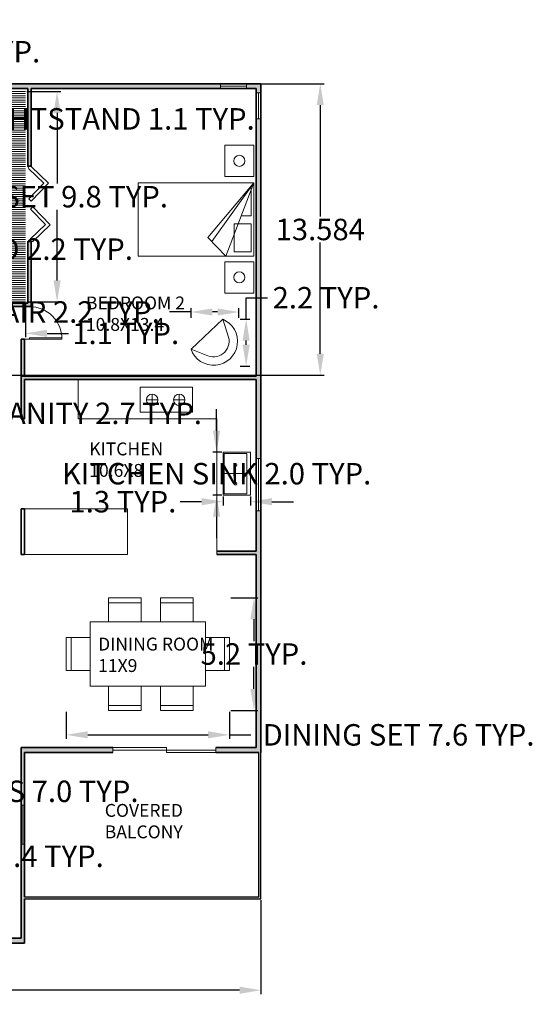
# Model space of a CAD drawing. Units: metres. Extents: x 25.1 to 96.1, y 24.3 to 71.3.
# Tile 5 of 5: x 72.2 to 96.1, y 24.9 to 70.8. Entities that reach past the tile are written whole.
import ezdxf

# ---------------------------------------------------------------- set-up
doc = ezdxf.new("R2010")
doc.units = ezdxf.units.M
doc.header["$MEASUREMENT"] = 0
for name, color, linetype, lineweight in [('A-AREA-IDEN', 1, 'Continuous', 18), ('A-EQPM', 163, 'Continuous', 18), ('A-FLOR-CASE', 8, 'Continuous', 18), ('A-FLOR-FIXT', 163, 'Continuous', 18), ('A-FLOR-RAIL', 7, 'Continuous', 25), ('A-GLAZ', 4, 'Continuous', 18), ('A-WALL', 7, 'Continuous', 35), ('A-WALL-PATT', 252, 'Continuous', 13), ('dimension', 80, 'Continuous', 18), ('door', 17, 'Continuous', 18), ('furniture', 163, 'Continuous', 18)]:
    doc.layers.add(name, color=color, linetype=linetype, lineweight=lineweight)
doc.styles.get("Standard").update_dxf_attribs({"font": 'arial.ttf'})
doc.dimstyles.get("Standard").update_dxf_attribs({"dimtxt": 1, "dimasz": 1, "dimexe": 0.18, "dimexo": 0.0625, "dimgap": 0.09, "dimtad": 0, "dimtih": 1, "dimtoh": 1, "dimdec": 1, "dimzin": 0, "dimdsep": 46, "dimtxsty": 'Standard', "dimcen": 0.09, "dimadec": 0, "dimazin": 0, "dimtfac": 1, "dimtdec": 1, "dimtofl": 0, "dimtmove": 0, "dimatfit": 3, "dimfxl": 1, "dimtolj": 1, "dimtzin": 0, "dimarcsym": 0})

# ---------------------------------------------------------------- blocks, each defined once
blk = doc.blocks.new('sink')
for points in [[(16.263, 3.026), (17.543, 3.026), (17.543, 1.019), (16.263, 1.019)], [(17.495, 2.968), (16.431, 2.968), (16.431, 2.028), (17.495, 2.028)], [(17.495, 2.028), (16.431, 2.028), (16.431, 1.081), (17.495, 1.081)]]:
    blk.add_lwpolyline(points, close=True)
for centre in [(16.963, 2.431), (16.961, 1.556)]:
    blk.add_circle(centre, 0.0675)
blk = doc.blocks.new('gas')
for p, q in [((20.28, 5.991), (20.28, 5.463)), ((21.546, 5.991), (21.546, 5.463)), ((20.016, 5.727), (20.544, 5.727)), ((21.282, 5.727), (21.81, 5.727))]:
    blk.add_line(p, q)
blk.add_lwpolyline([(19.729, 6.31), (22.157, 6.31), (22.157, 5.155), (19.729, 5.155)], close=True)
for centre in [(20.28, 5.727), (21.546, 5.727)]:
    blk.add_circle(centre, 0.264)
blk = doc.blocks.new('b')
for p, q in [((16.374, 15.368), (18.513, 12.83)), ((17.666, 11.96), (16.374, 15.368)), ((16.374, 15.368), (18.324, 12.637)), ((18.513, 12.83), (17.666, 11.96))]:
    blk.add_line(p, q)
for points in [[(16.362, 17.126), (17.718, 17.126), (17.718, 15.669), (16.362, 15.669)], [(16.374, 15.368), (21.762, 15.368), (21.762, 11.96), (16.374, 11.96)], [(16.486, 12.161), (17.289, 12.161), (17.289, 13.464), (16.486, 13.464)], [(16.362, 11.698), (17.718, 11.698), (17.718, 10.242), (16.362, 10.242)]]:
    blk.add_lwpolyline(points, close=True)
blk.add_lwpolyline([(16.564, 15.144), (16.486, 15.144), (16.486, 13.84), (16.953, 13.84)])
for centre in [(17.04, 16.398), (17.04, 10.97)]:
    blk.add_circle(centre, 0.259)
blk = doc.blocks.new('cc')
for p, q in [((17.83, 9.22), (17.545, 8.337)), ((17.83, 9.22), (19.307, 7.829)), ((19.307, 7.829), (18.516, 7.517))]:
    blk.add_line(p, q)
for radius, start, end in [(1.115, 112.1788, 341.2424), (0.721, 156.2062, 291.5475)]:
    blk.add_arc((18.251, 8.188), radius, start, end)
blk = doc.blocks.new('d')
for p, q in [((25.537, 16.335), (24.732, 15.559)), ((25.644, 16.224), (24.951, 15.555)), ((25.537, 16.335), (25.687, 16.335)), ((25.644, 16.224), (25.687, 16.335)), ((24.732, 15.559), (25.537, 14.725)), ((24.951, 15.555), (25.648, 14.833)), ((25.648, 14.833), (25.537, 14.725))]:
    blk.add_line(p, q)
blk = doc.blocks.new('f')
at = {"layer": 'furniture'}
for p, q in [((25.769, 19.917), (26.843, 19.917)), ((25.769, 19.817), (26.843, 19.817)), ((25.769, 19.717), (26.843, 19.717)), ((25.769, 19.617), (26.843, 19.617)), ((25.769, 19.517), (26.843, 19.517)), ((25.769, 19.417), (26.843, 19.417)), ((25.769, 19.317), (26.843, 19.317)), ((25.769, 19.217), (26.843, 19.217)), ((25.769, 19.117), (26.843, 19.117)), ((25.769, 19.017), (26.843, 19.017)), ((25.769, 18.917), (26.843, 18.917)), ((25.769, 18.817), (26.843, 18.817)), ((25.769, 18.717), (26.843, 18.717)), ((25.769, 18.617), (26.843, 18.617)), ((25.769, 18.517), (26.843, 18.517)), ((25.769, 18.417), (26.843, 18.417)), ((25.769, 18.317), (26.843, 18.317)), ((25.769, 18.217), (26.843, 18.217)), ((25.769, 18.117), (26.843, 18.117)), ((25.769, 18.017), (26.843, 18.017)), ((25.769, 17.917), (26.843, 17.917)), ((25.769, 17.817), (26.843, 17.817)), ((25.769, 17.717), (26.843, 17.717)), ((25.769, 17.617), (26.843, 17.617)), ((25.769, 17.517), (26.843, 17.517)), ((25.769, 17.417), (26.843, 17.417)), ((25.769, 17.317), (26.843, 17.317)), ((25.769, 17.217), (26.843, 17.217)), ((25.769, 17.117), (26.843, 17.117)), ((25.769, 17.017), (26.843, 17.017)), ((25.769, 16.917), (26.843, 16.917)), ((25.769, 16.817), (26.843, 16.817)), ((25.769, 16.717), (26.843, 16.717)), ((25.769, 16.617), (26.843, 16.617)), ((25.769, 16.517), (26.843, 16.517)), ((25.769, 16.417), (26.843, 16.417)), ((25.769, 16.317), (26.843, 16.317)), ((25.769, 16.217), (26.843, 16.217)), ((25.769, 16.117), (26.843, 16.117)), ((25.769, 16.017), (26.843, 16.017)), ((25.769, 15.917), (26.843, 15.917)), ((25.769, 15.817), (26.843, 15.817)), ((25.769, 15.717), (26.843, 15.717)), ((25.769, 15.617), (26.843, 15.617)), ((25.769, 15.517), (26.843, 15.517)), ((25.769, 15.417), (26.843, 15.417)), ((25.769, 15.317), (26.843, 15.317)), ((25.769, 15.217), (26.843, 15.217)), ((25.769, 15.117), (26.843, 15.117)), ((25.769, 15.017), (26.843, 15.017)), ((25.769, 14.917), (26.843, 14.917)), ((25.769, 14.817), (26.843, 14.817)), ((25.769, 14.717), (26.843, 14.717)), ((25.769, 14.617), (26.843, 14.617)), ((25.769, 14.517), (26.843, 14.517)), ((25.769, 14.417), (26.843, 14.417)), ((25.769, 14.317), (26.843, 14.317)), ((25.769, 14.217), (26.843, 14.217)), ((25.769, 14.117), (26.843, 14.117)), ((25.769, 14.017), (26.843, 14.017)), ((25.769, 13.917), (26.843, 13.917)), ((25.769, 13.817), (26.843, 13.817)), ((25.769, 13.717), (26.843, 13.717)), ((25.769, 13.617), (26.843, 13.617)), ((25.769, 13.517), (26.843, 13.517)), ((25.769, 13.417), (26.843, 13.417)), ((25.769, 13.317), (26.843, 13.317)), ((25.769, 13.217), (26.843, 13.217)), ((25.769, 13.117), (26.843, 13.117)), ((25.769, 13.017), (26.843, 13.017)), ((25.769, 12.917), (26.843, 12.917)), ((25.769, 12.817), (26.843, 12.817)), ((25.769, 12.717), (26.843, 12.717)), ((25.769, 12.617), (26.843, 12.617)), ((25.769, 12.517), (26.843, 12.517)), ((25.769, 12.417), (26.843, 12.417)), ((25.769, 12.317), (26.843, 12.317)), ((25.769, 12.217), (26.843, 12.217)), ((25.769, 12.117), (26.843, 12.117)), ((25.769, 12.017), (26.843, 12.017)), ((25.769, 11.917), (26.843, 11.917)), ((25.769, 11.817), (26.843, 11.817)), ((25.769, 11.717), (26.843, 11.717)), ((25.769, 11.617), (26.843, 11.617)), ((25.769, 11.517), (26.843, 11.517)), ((25.769, 11.417), (26.843, 11.417)), ((25.769, 11.317), (26.843, 11.317)), ((25.769, 11.217), (26.843, 11.217)), ((25.769, 11.117), (26.843, 11.117)), ((25.769, 11.017), (26.843, 11.017)), ((25.769, 10.917), (26.843, 10.917)), ((25.769, 10.817), (26.843, 10.817)), ((25.769, 10.717), (26.843, 10.717)), ((25.769, 10.617), (26.843, 10.617)), ((25.769, 10.517), (26.843, 10.517)), ((25.769, 10.417), (26.843, 10.417)), ((25.769, 10.317), (26.843, 10.317)), ((25.769, 10.217), (26.843, 10.217)), ((25.769, 10.117), (26.843, 10.117))]:
    blk.add_line(p, q, dxfattribs=at)
blk = doc.blocks.new('*U22')
for p, q in [((0, 0), (0, -6)), ((40, 0), (40, -6))]:
    blk.add_line(p, q)
blk.add_lwpolyline([(0, 0), (0, 40), (1.75, 40), (1.75, 0)], close=True)
blk.add_arc((0, 0), 40, 0, 90)
blk = doc.blocks.new('tttt')
for points in [[(21.475, -3.758), (19.715, -3.758), (19.715, -3.49), (21.475, -3.49)], [(24.267, -3.758), (22.507, -3.758), (22.507, -3.49), (24.267, -3.49)], [(19.715, -4.78), (21.475, -4.78), (21.475, -3.758), (19.715, -3.758)], [(22.507, -4.78), (24.267, -4.78), (24.267, -3.758), (22.507, -3.758)], [(18.746, -4.78), (24.929, -4.78), (24.929, -8.239), (18.746, -8.239)], [(17.724, -5.63), (17.724, -7.389), (17.456, -7.389), (17.456, -5.63)], [(18.746, -7.389), (18.746, -5.63), (17.724, -5.63), (17.724, -7.389)], [(24.929, -7.389), (24.929, -5.63), (25.951, -5.63), (25.951, -7.389)], [(25.951, -5.63), (25.951, -7.389), (26.219, -7.389), (26.219, -5.63)], [(19.715, -8.239), (21.475, -8.239), (21.475, -9.262), (19.715, -9.262)], [(22.507, -8.239), (24.267, -8.239), (24.267, -9.262), (22.507, -9.262)], [(21.475, -9.262), (19.715, -9.262), (19.715, -9.529), (21.475, -9.529)], [(24.267, -9.262), (22.507, -9.262), (22.507, -9.529), (24.267, -9.529)]]:
    blk.add_lwpolyline(points, close=True)
blk = doc.blocks.new('*D24')
at = {"layer": 'Defpoints', "color": 0, "transparency": 16777216}
for p in [(31.99, 29.798), (83.411, 29.798), (83.411, 25.547)]:
    blk.add_point(p, dxfattribs=at)
at = {"layer": 'dimension', "color": 0, "lineweight": -2, "transparency": 16777216}
for p, q in [((31.99, 29.735), (31.99, 25.367)), ((83.411, 29.735), (83.411, 25.367)), ((32.99, 25.547), (56.314, 25.547)), ((82.411, 25.547), (59.087, 25.547))]:
    blk.add_line(p, q, dxfattribs=at)
at = {"layer": 'dimension', "color": 0, "transparency": 16777216}
for points in [[(32.99, 25.713), (32.99, 25.38), (31.99, 25.547)], [(82.411, 25.713), (82.411, 25.38), (83.411, 25.547)]]:
    blk.add_solid(points, dxfattribs=at)
at = {"layer": 'dimension', "color": 0, "transparency": 16777216, "insert": (57.7, 25.547), "char_height": 1, "attachment_point": 5}
blk.add_mtext('\\A1;51.4', dxfattribs=at)
blk = doc.blocks.new('DOOR-BALCONY-SLIDING')
for p, q in [((0, 0.23), (2.501, 0.23)), ((2.501, 0.23), (2.501, 0)), ((2.501, 0), (4.797, 0))]:
    blk.add_line(p, q)
blk.add_lwpolyline([(4.797, 0.115), (4.797, 0.115), (0, 0.115), (0, 0.115)])
blk = doc.blocks.new('*D36')
at = {"layer": 'Defpoints', "color": 0, "transparency": 16777216}
for p in [(72.431, 67.419), (73.901, 67.419), (72.431, 57.619)]:
    blk.add_point(p, dxfattribs=at)
at = {"layer": 'dimension', "color": 0, "lineweight": -2, "transparency": 16777216}
for p, q in [((72.494, 67.419), (74.081, 67.419)), ((73.901, 66.419), (73.901, 63.126)), ((73.901, 58.619), (73.901, 61.912)), ((72.494, 57.619), (74.081, 57.619))]:
    blk.add_line(p, q, dxfattribs=at)
at = {"layer": 'dimension', "color": 0, "transparency": 16777216}
for points in [[(73.735, 66.419), (74.068, 66.419), (73.901, 67.419)], [(73.735, 58.619), (74.068, 58.619), (73.901, 57.619)]]:
    blk.add_solid(points, dxfattribs=at)
at = {"layer": 'dimension', "color": 0, "transparency": 16777216, "insert": (73.901, 62.519), "char_height": 1, "attachment_point": 5}
blk.add_mtext('\\A1;CLOSET 9.8 TYP.', dxfattribs=at)
blk = doc.blocks.new('*D37')
at = {"layer": 'Defpoints', "color": 0, "transparency": 16777216}
for p in [(71.357, 57.619), (72.431, 57.619), (72.431, 56.149)]:
    blk.add_point(p, dxfattribs=at)
at = {"layer": 'dimension', "color": 0, "lineweight": -2, "transparency": 16777216}
for p, q in [((71.357, 57.557), (71.357, 55.969)), ((72.431, 57.557), (72.431, 55.969)), ((70.357, 56.149), (69.357, 56.149)), ((73.431, 56.149), (74.431, 56.149))]:
    blk.add_line(p, q, dxfattribs=at)
at = {"layer": 'dimension', "color": 0, "transparency": 16777216}
for points in [[(70.357, 56.316), (70.357, 55.982), (71.357, 56.149)], [(73.431, 56.316), (73.431, 55.982), (72.431, 56.149)]]:
    blk.add_solid(points, dxfattribs=at)
at = {"layer": 'dimension', "color": 0, "transparency": 16777216, "insert": (77.102, 56.149), "char_height": 1, "attachment_point": 5}
blk.add_mtext('\\A1;1.1 TYP.', dxfattribs=at)
blk = doc.blocks.new('*D39')
at = {"layer": 'Defpoints', "color": 0, "transparency": 16777216}
for p in [(69.103, 30.788), (69.861, 30.788), (69.103, 28.392)]:
    blk.add_point(p, dxfattribs=at)
at = {"layer": 'dimension', "color": 0, "lineweight": -2, "transparency": 16777216}
for p, q in [((69.861, 30.788), (69.861, 31.788)), ((69.861, 31.788), (70.861, 31.788)), ((69.166, 30.788), (70.041, 30.788)), ((69.861, 29.392), (69.861, 29.788)), ((69.166, 28.392), (70.041, 28.392))]:
    blk.add_line(p, q, dxfattribs=at)
at = {"layer": 'dimension', "color": 0, "transparency": 16777216}
for points in [[(69.694, 29.788), (70.027, 29.788), (69.861, 30.788)], [(69.694, 29.392), (70.027, 29.392), (69.861, 28.392)]]:
    blk.add_solid(points, dxfattribs=at)
at = {"layer": 'dimension', "color": 0, "transparency": 16777216, "insert": (73.587, 31.788), "char_height": 1, "attachment_point": 5}
blk.add_mtext('\\A1;2.4 TYP.', dxfattribs=at)
blk = doc.blocks.new('*D42')
at = {"layer": 'Defpoints', "color": 0, "transparency": 16777216}
for p in [(81.341, 50.616), (81.642, 50.616), (81.642, 48.609)]:
    blk.add_point(p, dxfattribs=at)
at = {"layer": 'dimension', "color": 0, "lineweight": -2, "transparency": 16777216}
for p, q in [((81.341, 51.616), (81.341, 52.616)), ((81.579, 50.616), (81.161, 50.616)), ((81.579, 48.609), (81.161, 48.609)), ((81.341, 47.609), (81.341, 46.609))]:
    blk.add_line(p, q, dxfattribs=at)
at = {"layer": 'dimension', "color": 0, "transparency": 16777216}
for points in [[(81.174, 51.616), (81.507, 51.616), (81.341, 50.616)], [(81.174, 47.609), (81.507, 47.609), (81.341, 48.609)]]:
    blk.add_solid(points, dxfattribs=at)
at = {"layer": 'dimension', "color": 0, "transparency": 16777216, "insert": (81.341, 49.612), "char_height": 1, "attachment_point": 5}
blk.add_mtext('\\A1;KITCHEN SINK 2.0 TYP.', dxfattribs=at)
blk = doc.blocks.new('*D43')
at = {"layer": 'Defpoints', "color": 0, "transparency": 16777216}
for p in [(81.642, 48.609), (81.642, 48.308), (82.921, 48.609)]:
    blk.add_point(p, dxfattribs=at)
at = {"layer": 'dimension', "color": 0, "lineweight": -2, "transparency": 16777216}
for p, q in [((80.642, 48.308), (79.642, 48.308)), ((81.642, 48.546), (81.642, 48.128)), ((82.921, 48.546), (82.921, 48.128)), ((83.921, 48.308), (84.921, 48.308))]:
    blk.add_line(p, q, dxfattribs=at)
at = {"layer": 'dimension', "color": 0, "transparency": 16777216}
for points in [[(80.642, 48.474), (80.642, 48.141), (81.642, 48.308)], [(83.921, 48.474), (83.921, 48.141), (82.921, 48.308)]]:
    blk.add_solid(points, dxfattribs=at)
at = {"layer": 'dimension', "color": 0, "transparency": 16777216, "insert": (76.971, 48.308), "char_height": 1, "attachment_point": 5}
blk.add_mtext('\\A1;1.3 TYP.', dxfattribs=at)
blk = doc.blocks.new('*D48')
at = {"layer": 'Defpoints', "color": 0, "transparency": 16777216}
for p in [(80.148, 57.146), (80.148, 56.81), (82.383, 56.81)]:
    blk.add_point(p, dxfattribs=at)
at = {"layer": 'dimension', "color": 0, "lineweight": -2, "transparency": 16777216}
for p, q in [((80.148, 57.146), (79.148, 57.146)), ((80.148, 56.873), (80.148, 57.326)), ((81.383, 57.146), (81.148, 57.146)), ((82.383, 56.873), (82.383, 57.326))]:
    blk.add_line(p, q, dxfattribs=at)
at = {"layer": 'dimension', "color": 0, "transparency": 16777216}
for points in [[(81.148, 57.312), (81.148, 56.979), (80.148, 57.146)], [(81.383, 57.312), (81.383, 56.979), (82.383, 57.146)]]:
    blk.add_solid(points, dxfattribs=at)
at = {"layer": 'dimension', "color": 0, "transparency": 16777216, "insert": (74.068, 57.146), "char_height": 1, "attachment_point": 5}
blk.add_mtext('\\A1;CHAIR 2.2 TYP.', dxfattribs=at)
blk = doc.blocks.new('*D49')
at = {"layer": 'Defpoints', "color": 0, "transparency": 16777216}
for p in [(82.383, 56.81), (82.718, 56.81), (82.383, 54.621)]:
    blk.add_point(p, dxfattribs=at)
at = {"layer": 'dimension', "color": 0, "lineweight": -2, "transparency": 16777216}
for p, q in [((82.718, 56.81), (82.718, 57.81)), ((82.718, 57.81), (83.718, 57.81)), ((82.445, 56.81), (82.898, 56.81)), ((82.718, 55.621), (82.718, 55.81)), ((82.445, 54.621), (82.898, 54.621))]:
    blk.add_line(p, q, dxfattribs=at)
at = {"layer": 'dimension', "color": 0, "transparency": 16777216}
for points in [[(82.552, 55.81), (82.885, 55.81), (82.718, 56.81)], [(82.552, 55.621), (82.885, 55.621), (82.718, 54.621)]]:
    blk.add_solid(points, dxfattribs=at)
at = {"layer": 'dimension', "color": 0, "transparency": 16777216, "insert": (86.445, 57.81), "char_height": 1, "attachment_point": 5}
blk.add_mtext('\\A1;2.2 TYP.', dxfattribs=at)
blk = doc.blocks.new('*D54')
at = {"layer": 'Defpoints', "color": 0, "transparency": 16777216}
for p in [(63.784, 59.741), (66.011, 60.075), (66.011, 59.741)]:
    blk.add_point(p, dxfattribs=at)
at = {"layer": 'dimension', "color": 0, "lineweight": -2, "transparency": 16777216}
for p, q in [((63.784, 59.804), (63.784, 60.255)), ((66.011, 59.804), (66.011, 60.255)), ((64.784, 60.075), (65.011, 60.075)), ((66.011, 60.075), (67.011, 60.075))]:
    blk.add_line(p, q, dxfattribs=at)
at = {"layer": 'dimension', "color": 0, "transparency": 16777216}
for points in [[(64.784, 60.242), (64.784, 59.909), (63.784, 60.075)], [(65.011, 60.242), (65.011, 59.909), (66.011, 60.075)]]:
    blk.add_solid(points, dxfattribs=at)
at = {"layer": 'dimension', "color": 0, "transparency": 16777216, "insert": (72.424, 60.075), "char_height": 1, "attachment_point": 5}
blk.add_mtext('\\A1;BIFOLD 2.2 TYP.', dxfattribs=at)
blk = doc.blocks.new('*D60')
at = {"layer": 'Defpoints', "color": 0, "transparency": 16777216}
for p in [(66.561, 52.83), (69.281, 52.83), (69.281, 52.422)]:
    blk.add_point(p, dxfattribs=at)
at = {"layer": 'dimension', "color": 0, "lineweight": -2, "transparency": 16777216}
for p, q in [((66.561, 52.767), (66.561, 52.242)), ((69.281, 52.767), (69.281, 52.242)), ((67.561, 52.422), (68.281, 52.422)), ((69.281, 52.422), (70.281, 52.422))]:
    blk.add_line(p, q, dxfattribs=at)
at = {"layer": 'dimension', "color": 0, "transparency": 16777216}
for points in [[(67.561, 52.588), (67.561, 52.255), (66.561, 52.422)], [(68.281, 52.588), (68.281, 52.255), (69.281, 52.422)]]:
    blk.add_solid(points, dxfattribs=at)
at = {"layer": 'dimension', "color": 0, "transparency": 16777216, "insert": (75.742, 52.422), "char_height": 1, "attachment_point": 5}
blk.add_mtext('\\A1;VANITY 2.7 TYP.', dxfattribs=at)
blk = doc.blocks.new('*D66')
at = {"layer": 'Defpoints', "color": 0, "transparency": 16777216}
for p in [(74.329, 38.586), (81.943, 38.586), (81.943, 37.444)]:
    blk.add_point(p, dxfattribs=at)
at = {"layer": 'dimension', "color": 0, "lineweight": -2, "transparency": 16777216}
for p, q in [((74.329, 38.523), (74.329, 37.264)), ((81.943, 38.523), (81.943, 37.264)), ((75.329, 37.444), (80.943, 37.444)), ((81.943, 37.444), (82.943, 37.444))]:
    blk.add_line(p, q, dxfattribs=at)
at = {"layer": 'dimension', "color": 0, "transparency": 16777216}
for points in [[(75.329, 37.611), (75.329, 37.277), (74.329, 37.444)], [(80.943, 37.611), (80.943, 37.277), (81.943, 37.444)]]:
    blk.add_solid(points, dxfattribs=at)
at = {"layer": 'dimension', "color": 0, "transparency": 16777216, "insert": (89.827, 37.444), "char_height": 1, "attachment_point": 5}
blk.add_mtext('\\A1;DINING SET 7.6 TYP.', dxfattribs=at)
blk = doc.blocks.new('*D67')
at = {"layer": 'Defpoints', "color": 0, "transparency": 16777216}
for p in [(81.943, 43.833), (83.085, 43.833), (81.943, 38.586)]:
    blk.add_point(p, dxfattribs=at)
at = {"layer": 'dimension', "color": 0, "lineweight": -2, "transparency": 16777216}
for p, q in [((82.005, 43.833), (83.265, 43.833)), ((83.085, 42.833), (83.085, 41.81)), ((83.085, 39.586), (83.085, 40.609)), ((82.005, 38.586), (83.265, 38.586))]:
    blk.add_line(p, q, dxfattribs=at)
at = {"layer": 'dimension', "color": 0, "transparency": 16777216}
for points in [[(82.918, 42.833), (83.251, 42.833), (83.085, 43.833)], [(82.918, 39.586), (83.251, 39.586), (83.085, 38.586)]]:
    blk.add_solid(points, dxfattribs=at)
at = {"layer": 'dimension', "color": 0, "transparency": 16777216, "insert": (83.085, 41.21), "char_height": 1, "attachment_point": 5}
blk.add_mtext('\\A1;5.2 TYP.', dxfattribs=at)
blk = doc.blocks.new('*D70')
at = {"layer": 'Defpoints', "color": 0, "transparency": 16777216}
for p in [(65.697, 66.307), (66.786, 66.307), (66.786, 66.143)]:
    blk.add_point(p, dxfattribs=at)
at = {"layer": 'dimension', "color": 0, "lineweight": -2, "transparency": 16777216}
for p, q in [((64.697, 66.143), (63.697, 66.143)), ((65.697, 66.244), (65.697, 65.963)), ((66.786, 66.244), (66.786, 65.963)), ((67.786, 66.143), (68.786, 66.143))]:
    blk.add_line(p, q, dxfattribs=at)
at = {"layer": 'dimension', "color": 0, "transparency": 16777216}
for points in [[(64.697, 66.31), (64.697, 65.977), (65.697, 66.143)], [(67.786, 66.31), (67.786, 65.977), (66.786, 66.143)]]:
    blk.add_solid(points, dxfattribs=at)
at = {"layer": 'dimension', "color": 0, "transparency": 16777216, "insert": (76.214, 66.143), "char_height": 1, "attachment_point": 5}
blk.add_mtext('\\A1;NIGHTSTAND 1.1 TYP.', dxfattribs=at)
blk = doc.blocks.new('*D71')
at = {"layer": 'Defpoints', "color": 0, "transparency": 16777216}
for p in [(66.786, 67.273), (66.95, 67.273), (66.786, 66.307)]:
    blk.add_point(p, dxfattribs=at)
at = {"layer": 'dimension', "color": 0, "lineweight": -2, "transparency": 16777216}
for p, q in [((66.95, 68.273), (66.95, 69.273)), ((66.95, 69.273), (67.95, 69.273)), ((66.849, 67.273), (67.13, 67.273)), ((66.849, 66.307), (67.13, 66.307)), ((66.95, 65.307), (66.95, 64.307))]:
    blk.add_line(p, q, dxfattribs=at)
at = {"layer": 'dimension', "color": 0, "transparency": 16777216}
for points in [[(66.783, 68.273), (67.116, 68.273), (66.95, 67.273)], [(66.783, 65.307), (67.116, 65.307), (66.95, 66.307)]]:
    blk.add_solid(points, dxfattribs=at)
at = {"layer": 'dimension', "color": 0, "transparency": 16777216, "insert": (70.621, 69.273), "char_height": 1, "attachment_point": 5}
blk.add_mtext('\\A1;1.0 TYP.', dxfattribs=at)
blk = doc.blocks.new('*D72')
at = {"layer": 'Defpoints', "color": 0, "transparency": 16777216}
for p in [(54.201, 35.864), (61.201, 35.864), (61.201, 34.814)]:
    blk.add_point(p, dxfattribs=at)
at = {"layer": 'dimension', "color": 0, "lineweight": -2, "transparency": 16777216}
for p, q in [((54.201, 35.801), (54.201, 34.634)), ((61.201, 35.801), (61.201, 34.634)), ((55.201, 34.814), (60.201, 34.814)), ((61.201, 34.814), (62.201, 34.814))]:
    blk.add_line(p, q, dxfattribs=at)
at = {"layer": 'dimension', "color": 0, "transparency": 16777216}
for points in [[(55.201, 34.98), (55.201, 34.647), (54.201, 34.814)], [(60.201, 34.98), (60.201, 34.647), (61.201, 34.814)]]:
    blk.add_solid(points, dxfattribs=at)
at = {"layer": 'dimension', "color": 0, "transparency": 16777216, "insert": (70.311, 34.814), "char_height": 1, "attachment_point": 5}
blk.add_mtext('\\A1;STAIR FLIGHTS 7.0 TYP.', dxfattribs=at)
blk = doc.blocks.new('*D85')
at = {"layer": 'Defpoints', "color": 0, "transparency": 16777216}
for p in [(54.201, 67.782), (86.176, 67.782), (54.201, 54.198)]:
    blk.add_point(p, dxfattribs=at)
at = {"layer": 'dimension', "color": 0, "lineweight": -2, "transparency": 16777216}
for p, q in [((54.263, 67.782), (86.356, 67.782)), ((86.176, 66.782), (86.176, 61.59)), ((86.176, 55.198), (86.176, 60.389)), ((54.263, 54.198), (86.356, 54.198))]:
    blk.add_line(p, q, dxfattribs=at)
at = {"layer": 'dimension', "color": 0, "transparency": 16777216}
for points in [[(86.009, 66.782), (86.342, 66.782), (86.176, 67.782)], [(86.009, 55.198), (86.342, 55.198), (86.176, 54.198)]]:
    blk.add_solid(points, dxfattribs=at)
at = {"layer": 'dimension', "color": 0, "transparency": 16777216, "insert": (86.176, 60.99), "char_height": 1, "attachment_point": 5}
blk.add_mtext('\\A1;13.584', dxfattribs=at)

msp = doc.modelspace()

# ---------------------------------------------------------------- hatches: boundary and pattern name
at = {"layer": 'A-WALL-PATT'}
h = msp.add_hatch(color=256, dxfattribs=at)
h.dxf.hatch_style = 1
h.paths.add_polyline_path([(72.6908, 67.5516), (81.5153, 67.5516), (81.5153, 67.7816), (70.1857, 67.7816), (70.1857, 67.5516), (71.1708, 67.5516), (71.1708, 57.5516), (70.8915, 57.5516), (70.8915, 57.4016), (72.2308, 57.4016), (72.6908, 57.4016), (72.6908, 60.436), (72.6185, 60.436), (72.5408, 60.436), (72.5408, 57.5516), (71.3208, 57.5516), (71.3208, 67.5516), (72.5408, 67.5516), (72.5408, 63.9324), (72.6908, 63.9324)])
h.paths.add_polyline_path([(83.4108, 67.7816), (82.7353, 67.7816), (82.7353, 67.5516), (83.1808, 67.5516), (83.1808, 67.3623), (83.4108, 67.3623)])
h = msp.add_hatch(color=256, dxfattribs=at)
h.dxf.hatch_style = 1
h.paths.add_polyline_path([(83.4108, 66.1423), (83.1808, 66.1423), (83.1808, 54.1516), (72.2308, 54.1516), (72.2308, 54.0016), (72.2308, 52.1716), (72.3808, 52.1716), (72.3808, 52.7816), (72.3808, 54.0016), (83.1808, 54.0016), (83.1808, 50.3184), (83.4108, 50.3184), (83.4108, 54.0016)])
h.paths.add_polyline_path([(72.3808, 55.8816), (72.2308, 55.8816), (72.2308, 54.1516), (72.3808, 54.1516)], flags=17)
h = msp.add_hatch(color=256, dxfattribs=at)
h.dxf.hatch_style = 1
h.paths.add_polyline_path([(83.4108, 47.8784), (83.1808, 47.8784), (83.1808, 46.0016), (81.3508, 46.0016), (81.3508, 45.8516), (83.1808, 45.8516), (83.1808, 36.8516), (81.298, 36.8516), (81.298, 36.6216), (83.3108, 36.6216), (83.3108, 29.8975), (72.3808, 29.8975), (72.3808, 32.3495), (72.2308, 32.3495), (72.2308, 27.9675), (68.6208, 27.9675), (68.6208, 27.7375), (72.3808, 27.7375), (72.3808, 29.7975), (83.4108, 29.7975), (83.4108, 36.6216)])
h.paths.add_polyline_path([(76.5012, 36.8516), (72.2308, 36.8516), (72.2308, 34.1695), (72.3808, 34.1695), (72.3808, 36.6216), (76.5012, 36.6216)], flags=17)
h.paths.add_polyline_path([(61.4308, 32.2335), (61.2008, 32.2335), (61.2008, 27.7375), (61.4308, 27.7375), (64.9608, 27.7375), (64.9608, 27.9675), (61.4308, 27.9675)])

# ---------------------------------------------------------------- linework, layer by layer
at = {"layer": 'A-FLOR-CASE'}
for p, q in [((74.8866, 52.1716), (74.8866, 54.0016)), ((74.8866, 52.1716), (81.3508, 52.1716)), ((81.3508, 52.1716), (81.3508, 45.8516)), ((72.3808, 47.9816), (77.1808, 47.9816)), ((77.1808, 47.9816), (77.1808, 45.8516)), ((72.3808, 45.8516), (77.1808, 45.8516))]:
    msp.add_line(p, q, dxfattribs=at)
at = {"layer": 'A-FLOR-RAIL'}
for p, q in [((83.3108, 29.8975), (83.3108, 36.6216)), ((83.4108, 29.7975), (83.4108, 36.6216)), ((72.3808, 29.8975), (83.3108, 29.8975)), ((72.3808, 29.7975), (83.4108, 29.7975))]:
    msp.add_line(p, q, dxfattribs=at)
at = {"layer": 'A-GLAZ'}
for p, q in [((81.5153, 67.5516), (81.5153, 67.7816)), ((81.5153, 67.6666), (82.7353, 67.6666)), ((82.7353, 67.5516), (82.7353, 67.7816)), ((83.1808, 67.3623), (83.4108, 67.3623)), ((83.2958, 66.1423), (83.2958, 67.3623)), ((83.1808, 66.1423), (83.4108, 66.1423)), ((83.4108, 50.3184), (83.1808, 50.3184)), ((83.2958, 50.3184), (83.2958, 47.8784)), ((83.4108, 47.8784), (83.1808, 47.8784)), ((72.3808, 34.1695), (72.2308, 34.1695)), ((72.3058, 32.3495), (72.3058, 34.1695)), ((72.3808, 32.3495), (72.2308, 32.3495))]:
    msp.add_line(p, q, dxfattribs=at)
at = {"layer": 'A-WALL'}
for p, q in [((58.8908, 67.7816), (83.4108, 67.7816)), ((71.3208, 67.5516), (72.5408, 67.5516)), ((72.5408, 67.5516), (72.5408, 63.9324)), ((72.6908, 67.5516), (72.6908, 63.9324)), ((72.6908, 67.5516), (83.1808, 67.5516)), ((83.1808, 67.5516), (83.1808, 54.1516)), ((83.4108, 67.7816), (83.4108, 54.0016)), ((72.5408, 63.9324), (72.6908, 63.9324)), ((72.6908, 60.436), (72.5408, 60.436)), ((72.5408, 60.436), (72.5408, 57.5516)), ((72.6908, 60.436), (72.6908, 57.4016)), ((70.8915, 57.4016), (72.2308, 57.4016)), ((71.3208, 57.5516), (72.5408, 57.5516)), ((72.2308, 57.4016), (72.6908, 57.4016)), ((72.2308, 55.8816), (72.2308, 54.0016)), ((72.2308, 55.8816), (72.3808, 55.8816)), ((72.3808, 55.8816), (72.3808, 54.1516)), ((72.2308, 54.1516), (83.1808, 54.1516)), ((72.2308, 54.0016), (72.2308, 52.1716)), ((72.3808, 54.0016), (83.1808, 54.0016)), ((72.3808, 54.0016), (72.3808, 52.7816)), ((83.1808, 54.0016), (83.1808, 46.0016)), ((83.4108, 54.0016), (83.4108, 36.6216)), ((72.3808, 52.7816), (72.3808, 52.1716)), ((72.3808, 52.1716), (72.2308, 52.1716)), ((72.2308, 47.9816), (72.3808, 47.9816)), ((72.2308, 47.9816), (72.2308, 45.8516)), ((72.3808, 47.9816), (72.3808, 45.8516)), ((81.3508, 46.0016), (83.1808, 46.0016)), ((72.2308, 45.8516), (72.3808, 45.8516)), ((81.3508, 45.8516), (83.1808, 45.8516)), ((83.1808, 45.8516), (83.1808, 36.8516)), ((72.2308, 36.8516), (72.2308, 27.9675)), ((76.5012, 36.8516), (72.2308, 36.8516)), ((81.298, 36.8516), (83.1808, 36.8516)), ((72.3808, 36.6216), (76.5012, 36.6216)), ((72.3808, 36.6216), (72.3808, 29.8975)), ((81.298, 36.6216), (83.3108, 36.6216)), ((72.3808, 29.7975), (72.3808, 27.7375)), ((61.2008, 27.7375), (72.3808, 27.7375)), ((61.4308, 27.9675), (72.2308, 27.9675))]:
    msp.add_line(p, q, dxfattribs=at)
at = {"layer": 'door'}
for p, q in [((76.5012, 36.8516), (76.5012, 36.6216)), ((81.298, 36.6216), (81.298, 36.8516))]:
    msp.add_line(p, q, dxfattribs=at)

# ---------------------------------------------------------------- block references
at = {"layer": 'A-EQPM'}
msp.add_blockref('gas', (58.054, 47.327), dxfattribs=at)
at = {"layer": 'A-FLOR-CASE'}
msp.add_blockref('f', (45.5881, 47.5021), dxfattribs=at)
at = {"layer": 'A-FLOR-FIXT', "xscale": -1}
msp.add_blockref('sink', (99.1844, 47.5898), dxfattribs=at)
at = {"layer": 'door', "xscale": -1}
msp.add_blockref('d', (98.2302, 47.5898), dxfattribs=at)
at = {"layer": 'door', "rotation": 180}
msp.add_blockref('d', (98.3052, 76.7713), dxfattribs=at)
at = {"layer": 'door', "xscale": -0.0379497194996768, "yscale": 0.0379497194996768, "zscale": 0.0379497194996768, "rotation": 269.9999999999993}
msp.add_blockref('*U22', (72.6085, 55.8816), dxfattribs=at)
at = {"layer": 'door'}
msp.add_blockref('DOOR-BALCONY-SLIDING', (76.5014, 36.622), dxfattribs=at)
at = {"layer": 'furniture', "xscale": -1}
for name, p in [('b', (99.4439, 47.7883)), ('cc', (99.4545, 47.5898))]:
    msp.add_blockref(name, p, dxfattribs=at)
at = {"layer": 'furniture', "xscale": 0.8688370319284477, "yscale": 0.8688370319284477, "zscale": 0.8688370319284477}
msp.add_blockref('tttt', (59.1628, 46.8655), dxfattribs=at)

# ---------------------------------------------------------------- texts
at = {"layer": 'A-AREA-IDEN', "char_height": 0.6, "attachment_point": 1}
for s, width, insert in [('BEDROOM 2\\P10.8X13.4', 5.007262, (75.2457, 57.8667)), ('KITCHEN\\P10.6X8', 5.007262, (75.4008, 51.0655)), ('DINING ROOM\\P11X9', 7.366073, (75.8147, 41.9738)), ('COVERED\\PBALCONY', 5.007262, (76.1244, 34.2251))]:
    msp.add_mtext_dynamic_manual_height_columns(s, width=width, gutter_width=1, heights=[0], dxfattribs=dict(at, insert=insert))

# ---------------------------------------------------------------- dimensions: what is measured, and where the dimension line sits
at = {"layer": 'dimension'}
for base, p1, p2, angle, text, picture, middle in [((66.9497, 67.2729), (66.7863, 66.3066), (66.7863, 67.2729), 90, '<> TYP.', '*D71', (70.6206, 69.2729)), ((73.9012, 67.4191), (72.4312, 57.6191), (72.4312, 67.4191), 90, 'CLOSET <> TYP.', '*D36', (73.9012, 62.5191)), ((80.1479, 57.1455), (82.383, 56.8102), (80.1479, 56.8102), 180, 'CHAIR <> TYP.', '*D48', (74.0685, 57.1455)), ((82.7183, 56.8102), (82.383, 54.6211), (82.383, 56.8102), 90, '<> TYP.', '*D49', (86.4447, 57.8102)), ((81.3406, 50.6156), (81.6416, 48.6086), (81.6416, 50.6156), 90, 'KITCHEN SINK <> TYP.', '*D42', (81.3406, 49.6121)), ((81.6416, 48.3075), (82.9212, 48.6086), (81.6416, 48.6086), 180, '<> TYP.', '*D43', (76.9708, 48.3075)), ((83.0847, 43.8331), (81.9427, 38.586), (81.9427, 43.8331), 90, '<> TYP.', '*D67', (83.0847, 41.2096)), ((69.8605, 30.788), (69.1034, 28.392), (69.1034, 30.788), 90, '<> TYP.', '*D39', (73.587, 31.788))]:
    dim = msp.add_linear_dim(base=base, p1=p1, p2=p2, angle=angle, text=text, dimstyle='Standard', override={"dimdec": 1, "dimlfac": 1, "dimrnd": 0, "dimzin": 0, "dimdsep": 46, "dimlunit": 2}, dxfattribs=at)
    dim.commit()
    dim.dimension.update_dxf_attribs({"geometry": picture, "text_midpoint": middle})
for base, p1, p2, text, picture, middle in [((66.7863, 66.1432), (65.6965, 66.3066), (66.7863, 66.3066), 'NIGHTSTAND <> TYP.', '*D70', (76.2143, 66.1432)), ((66.0112, 60.0752), (63.7844, 59.7412), (66.0112, 59.7412), 'BIFOLD <> TYP.', '*D54', (72.4239, 60.0752)), ((72.4312, 56.1491), (71.3574, 57.6191), (72.4312, 57.6191), '<> TYP.', '*D37', (77.1021, 56.1491)), ((69.2808, 52.4216), (66.5611, 52.8295), (69.2808, 52.8295), 'VANITY <> TYP.', '*D60', (75.7415, 52.4216)), ((81.9427, 37.4439), (74.3291, 38.586), (81.9427, 38.586), 'DINING SET <> TYP.', '*D66', (89.827, 37.4439)), ((61.2008, 34.8135), (54.2008, 35.8635), (61.2008, 35.8635), 'STAIR FLIGHTS <> TYP.', '*D72', (70.3109, 34.8135))]:
    dim = msp.add_linear_dim(base=base, p1=p1, p2=p2, text=text, dimstyle='Standard', override={"dimdec": 1, "dimlfac": 1, "dimrnd": 0, "dimzin": 0, "dimdsep": 46, "dimlunit": 2}, dxfattribs=at)
    dim.commit()
    dim.dimension.update_dxf_attribs({"geometry": picture, "text_midpoint": middle})
dim = msp.add_linear_dim(base=(86.1758, 67.7816), p1=(54.2008, 54.1975), p2=(54.2008, 67.7816), angle=90, dimstyle='Standard', override={"dimdec": 3, "dimlfac": 1, "dimrnd": 0, "dimzin": 0, "dimdsep": 46, "dimlunit": 2}, dxfattribs=at)
dim.commit()
dim.dimension.update_dxf_attribs({"geometry": '*D85', "text_midpoint": (86.1758, 60.9895)})
dim = msp.add_linear_dim(base=(83.4108, 25.5466), p1=(31.9902, 29.7975), p2=(83.4108, 29.7975), dimstyle='Standard', override={"dimclrd": 0, "dimclre": 0, "dimclrt": 0}, dxfattribs=at)
dim.commit()
dim.dimension.update_dxf_attribs({"geometry": '*D24', "text_midpoint": (57.7005, 25.5466)})

doc.saveas('drawing.dxf')
